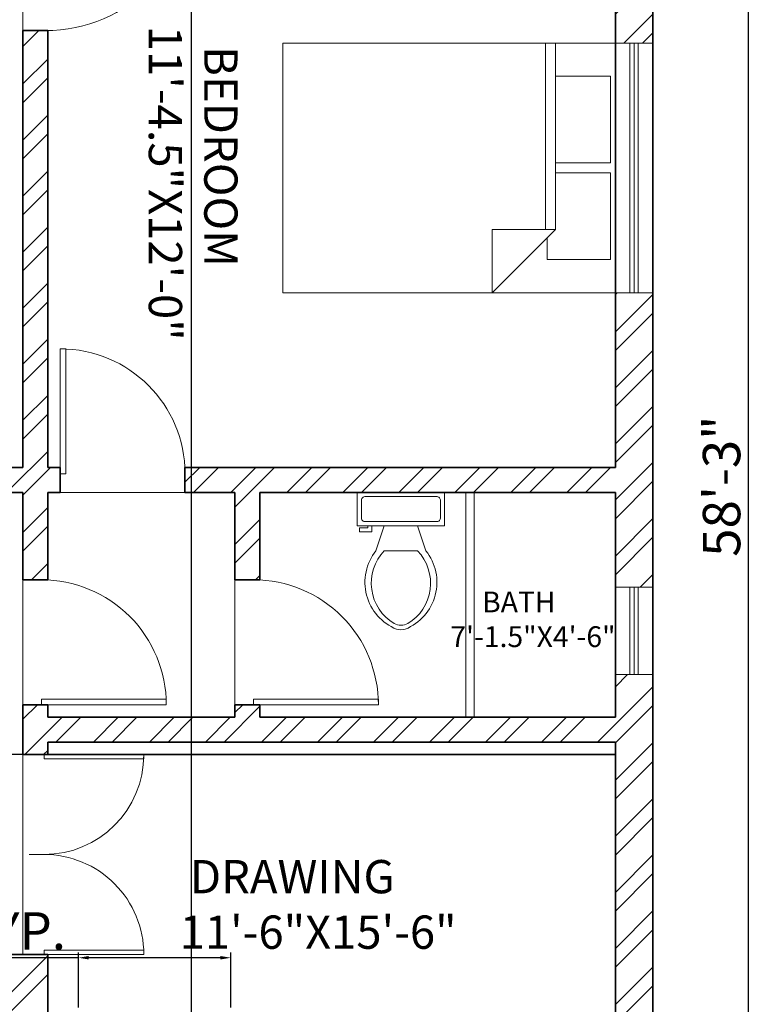
# Model space of a CAD drawing. Units: inches. Extents: x 287 to 905, y 1151 to 2037.
# Tile 4 of 5: x 646 to 822, y 1503 to 1739. Entities that reach past the tile are written whole.
import ezdxf

# ---------------------------------------------------------------- set-up
doc = ezdxf.new("R2010")
doc.units = ezdxf.units.IN
for name, color, linetype, lineweight in [('A-ANNO-DIMS', 2, 'Continuous', 18), ('A-AREA-IDEN', 7, 'Continuous', 18), ('A-DOOR', 4, 'Continuous', 18), ('A-FLOR-FIXT', 8, 'Continuous', 18), ('A-FURN', 9, 'Continuous', 18), ('A-WALL', 7, 'Continuous', 35), ('A-WALL-PATT', 252, 'Continuous', 13)]:
    doc.layers.add(name, color=color, linetype=linetype, lineweight=lineweight)
doc.layers.add('A-GLAZ', color=244, linetype='Continuous', lineweight=18, true_color=0x991b1e)
doc.layers.add('L-PLNT-PATT', color=116, linetype='Continuous', lineweight=13, true_color=0x136734)
doc.styles.get("Standard").update_dxf_attribs({"font": 'arial.ttf'})
doc.dimstyles.new('ISO-25', dxfattribs={"dimtxt": 9, "dimasz": 2.5, "dimexe": 1.25, "dimexo": 0.625, "dimtad": 1, "dimlunit": 3, "dimtxsty": 'Standard', "dimcen": 2.5, "dimadec": 0, "dimazin": 0, "dimtfac": 1, "dimtmove": 0, "dimatfit": 3, "dimfxl": 1, "dimarcsym": 0})

# ---------------------------------------------------------------- blocks, each defined once
blk = doc.blocks.new('*U2')
for p, q in [((0, 0), (0, -6)), ((40, 0), (40, -6))]:
    blk.add_line(p, q)
blk.add_lwpolyline([(0, 0), (0, 40), (1.75, 40), (1.75, 0)], close=True)
blk.add_arc((0, 0), 40, 0, 90)
blk = doc.blocks.new('*U3')
for p, q in [((0, 0), (0, -6)), ((-40, 0), (-40, -6))]:
    blk.add_line(p, q)
blk.add_lwpolyline([(0, 0), (0, 40), (-1.75, 40), (-1.75, 0)], close=True)
blk.add_arc((0, 0), 40, 90, 180)
blk = doc.blocks.new('*U6')
for p, q in [((0, 0), (0, -6)), ((40, 0), (40, -6))]:
    blk.add_line(p, q)
blk.add_lwpolyline([(0, 0), (0, 40), (1.75, 40), (1.75, 0)], close=True)
blk.add_arc((0, 0), 40, 0, 90)
blk = doc.blocks.new('Bed - Queen')
for p, q in [((0, -80.00003), (0, 0)), ((0, 0), (59.99999, 0)), ((59.99999, 0), (59.99999, -80.00003)), ((7.99999, -1.2), (28.79998, -1.2)), ((7.99999, -14.4), (7.99999, -1.2)), ((28.79998, -1.2), (28.79998, -14.4)), ((31.19999, -1.2), (51.99999, -1.2)), ((31.19999, -14.4), (31.19999, -1.2)), ((51.99999, -1.2), (51.99999, -16.4)), ((0, -14.4), (44.8, -14.4)), ((59.99999, -29.6), (44.8, -14.4)), ((44.8, -14.4), (44.8, -29.6)), ((51.99999, -16.4), (46.79936, -16.4)), ((44.8, -16.8), (0, -16.8)), ((44.8, -29.6), (59.99999, -29.6)), ((59.99999, -80.00003), (0, -80.00003))]:
    blk.add_line(p, q)
blk = doc.blocks.new('*D14')
at = {"layer": 'A-ANNO-DIMS', "color": 0, "lineweight": -2, "transparency": 16777216}
for p, q in [((798.48, 1976.83), (822.01, 1976.83)), ((820.76, 1974.33), (820.76, 1280.33)), ((798.48, 1277.83), (822.01, 1277.83))]:
    blk.add_line(p, q, dxfattribs=at)
at = {"layer": 'A-ANNO-DIMS', "color": 0, "transparency": 16777216}
for points in [[(820.35, 1974.33), (821.18, 1974.33), (820.76, 1976.83)], [(820.35, 1280.33), (821.18, 1280.33), (820.76, 1277.83)]]:
    blk.add_solid(points, dxfattribs=at)
at = {"layer": 'Defpoints', "color": 0, "transparency": 16777216}
for p in [(797.86, 1976.83), (797.86, 1277.83), (820.76, 1277.83)]:
    blk.add_point(p, dxfattribs=at)
at = {"layer": 'A-ANNO-DIMS', "color": 0, "transparency": 16777216, "insert": (815.54, 1627.33), "char_height": 9, "attachment_point": 5, "rotation": 90}
blk.add_mtext('58\'-3"', dxfattribs=at)
blk = doc.blocks.new('*U12')
for p, q in [((9.5, -6), (9.5, -2)), ((-10, -8.5), (-8, -8.5)), ((-10, -9.5), (-10, -8.5)), ((-8, -8.5), (-8, -8)), ((-7, -8), (-7, -9.5)), ((-4, -8), (-6, -14)), ((4, -8), (6, -14)), ((-7, -9.5), (-10, -9.5)), ((4, -14), (-4, -14))]:
    blk.add_line(p, q)
blk.add_lwpolyline([(10.5, -8), (10.5, 0), (-10.5, 0), (-10.5, -8)], close=True)
for points in [[(-9.5, -2), (-9.5, -6)], [(8.5, -1), (-8.5, -1)], [(-8.5, -7), (8.5, -7)]]:
    blk.add_lwpolyline(points)
for centre, radius, start, end in [((-8.62, -1.88), 0.884, 81.8699, 188.1301), ((8.62, -1.88), 0.884, 351.8699, 98.1301), ((-8.62, -6.12), 0.884, 171.8699, 278.1301), ((8.62, -6.12), 0.884, 261.8699, 8.1301), ((3.52, -21.58), 12.17, 141.4691, 247.9714), ((4.2, -21.82), 11.33, 136.3677, 238.9468), ((-3.52, -21.58), 12.17, 292.0284, 38.5307), ((-4.2, -21.82), 11.33, 301.053, 43.6321), ((0, -27.88), 4, 245.7318, 294.2682), ((0, -29), 4, 254.8605, 285.1395)]:
    blk.add_arc(centre, radius, start, end)
blk = doc.blocks.new('WIN-21IN')
for p, q in [((-10.5, 1), (10.5, 1)), ((-10.5, 0), (10.5, 0)), ((-10.5, -1), (10.5, -1))]:
    blk.add_line(p, q)
blk.add_lwpolyline([(-10.5, 4.5), (10.5, 4.5), (10.5, -4.5), (-10.5, -4.5)], close=True)
blk = doc.blocks.new('WIN-60IN')
for p, q in [((-1, 30), (-1, -30)), ((0, 30), (0, -30)), ((1, 30), (1, -30))]:
    blk.add_line(p, q)
blk.add_lwpolyline([(-4.5, 30), (4.5, 30), (4.5, -30), (-4.5, -30)], close=True)
blk = doc.blocks.new('*D25')
at = {"layer": 'A-ANNO-DIMS', "color": 0, "lineweight": -2, "transparency": 16777216}
for p, q in [((659.72, 1502.05), (659.72, 1515.27)), ((696.39, 1502.05), (696.39, 1515.27)), ((659.72, 1514.02), (580.15, 1514.02)), ((693.89, 1514.02), (662.22, 1514.02))]:
    blk.add_line(p, q, dxfattribs=at)
at = {"layer": 'A-ANNO-DIMS', "color": 0, "transparency": 16777216}
for points in [[(662.22, 1514.44), (662.22, 1513.61), (659.72, 1514.02)], [(693.89, 1514.44), (693.89, 1513.61), (696.39, 1514.02)]]:
    blk.add_solid(points, dxfattribs=at)
at = {"layer": 'Defpoints', "color": 0, "transparency": 16777216}
for p in [(659.72, 1514.02), (659.72, 1501.42), (696.39, 1501.42)]:
    blk.add_point(p, dxfattribs=at)
at = {"layer": 'A-ANNO-DIMS', "color": 0, "transparency": 16777216, "insert": (618.68, 1519.3), "char_height": 9, "attachment_point": 5}
blk.add_mtext('3\'-0 1/2" TYP.', dxfattribs=at)
blk = doc.blocks.new('*D35')
at = {"layer": 'A-ANNO-DIMS', "color": 0, "lineweight": -2, "transparency": 16777216}
for p, q in [((651.73, 1562.83), (370.73, 1562.83)), ((371.98, 1517.33), (371.98, 1560.33)), ((651.73, 1514.83), (370.73, 1514.83))]:
    blk.add_line(p, q, dxfattribs=at)
at = {"layer": 'A-ANNO-DIMS', "color": 0, "transparency": 16777216}
for points in [[(371.57, 1560.33), (372.4, 1560.33), (371.98, 1562.83)], [(371.57, 1517.33), (372.4, 1517.33), (371.98, 1514.83)]]:
    blk.add_solid(points, dxfattribs=at)
at = {"layer": 'Defpoints', "color": 0, "transparency": 16777216}
for p in [(371.98, 1562.83), (652.36, 1562.83), (652.36, 1514.83)]:
    blk.add_point(p, dxfattribs=at)
at = {"layer": 'A-ANNO-DIMS', "color": 0, "transparency": 16777216, "insert": (366.76, 1538.83), "char_height": 9, "attachment_point": 5, "rotation": 90}
blk.add_mtext('4\'-0"', dxfattribs=at)
blk = doc.blocks.new('*D37')
at = {"layer": 'A-ANNO-DIMS', "color": 0, "lineweight": -2, "transparency": 16777216}
for p, q in [((524.86, 1967.21), (524.86, 1157.65)), ((686.86, 1967.21), (686.86, 1157.65)), ((527.36, 1158.9), (684.36, 1158.9))]:
    blk.add_line(p, q, dxfattribs=at)
at = {"layer": 'A-ANNO-DIMS', "color": 0, "transparency": 16777216}
for points in [[(527.36, 1159.32), (527.36, 1158.49), (524.86, 1158.9)], [(684.36, 1159.32), (684.36, 1158.49), (686.86, 1158.9)]]:
    blk.add_solid(points, dxfattribs=at)
at = {"layer": 'Defpoints', "color": 0, "transparency": 16777216}
for p in [(524.86, 1967.83), (686.86, 1967.83), (686.86, 1158.9)]:
    blk.add_point(p, dxfattribs=at)
at = {"layer": 'A-ANNO-DIMS', "color": 0, "transparency": 16777216, "insert": (605.86, 1164.13), "char_height": 9, "attachment_point": 5}
blk.add_mtext('13\'-6"', dxfattribs=at)

msp = doc.modelspace()

# ---------------------------------------------------------------- hatches: boundary and pattern name
at = {"layer": 'A-WALL-PATT'}
h = msp.add_hatch(dxfattribs=at)
h.set_pattern_fill('ANSI32', color=256)
h.paths.add_polyline_path([(604.357, 1511.833), (519.857, 1511.833), (519.857, 1625.833), (607.357, 1625.833), (607.357, 1631.833), (510.857, 1631.833), (510.857, 1625.833), (513.857, 1625.833), (513.857, 1511.833), (496.063, 1511.833), (496.063, 1502.833), (604.357, 1502.833)])
h.paths.add_polyline_path([(652.357, 1511.833), (652.357, 1514.833), (643.357, 1514.833), (643.357, 1511.833), (640.357, 1511.833), (640.357, 1505.833), (643.357, 1505.833), (643.357, 1370.833), (690.607, 1370.833), (690.607, 1379.833), (652.357, 1379.833)])
h.paths.add_polyline_path([(797.857, 1582.055), (788.857, 1582.055), (788.857, 1571.833), (703.357, 1571.833), (703.357, 1574.833), (697.357, 1574.833), (697.357, 1571.833), (652.357, 1571.833), (652.357, 1574.833), (646.357, 1574.833), (646.357, 1562.833), (652.357, 1562.833), (652.357, 1565.833), (788.857, 1565.833), (788.857, 1379.833), (750.607, 1379.833), (750.607, 1370.833), (797.857, 1370.833)])
h.paths.add_polyline_path([(797.857, 1673.833), (788.857, 1673.833), (788.857, 1631.833), (685.357, 1631.833), (685.357, 1625.833), (697.357, 1625.833), (697.357, 1604.833), (703.357, 1604.833), (703.357, 1625.833), (788.857, 1625.833), (788.857, 1603.055), (797.857, 1603.055)])
h.paths.add_polyline_path([(797.857, 1976.833), (751.357, 1976.833), (751.357, 1967.833), (788.857, 1967.833), (788.857, 1919.833), (785.857, 1919.833), (785.857, 1913.833), (788.857, 1913.833), (788.857, 1781.833), (654.342, 1781.833), (643.328, 1792.848), (639.085, 1788.605), (645.857, 1781.833), (645.857, 1775.833), (646.357, 1775.833), (646.357, 1772.833), (652.357, 1772.833), (652.357, 1775.833), (788.857, 1775.833), (788.857, 1733.833), (797.857, 1733.833)])
h.paths.add_polyline_path([(755.857, 1919.833), (692.857, 1919.833), (692.857, 1967.833), (730.357, 1967.833), (730.357, 1976.833), (473.78, 1976.833), (473.78, 1967.833), (518.857, 1967.833), (518.857, 1919.833), (455.857, 1919.833), (455.857, 1913.833), (567.857, 1913.833), (567.857, 1919.833), (524.857, 1919.833), (524.857, 1967.833), (686.857, 1967.833), (686.857, 1919.833), (639.857, 1919.833), (639.857, 1913.833), (755.857, 1913.833)])
h.paths.add_polyline_path([(606.857, 1913.833), (609.857, 1913.833), (609.857, 1919.833), (597.857, 1919.833), (597.857, 1913.833), (600.857, 1913.833), (600.857, 1829.319), (589.842, 1818.304), (594.085, 1814.061), (600.857, 1820.833), (600.857, 1781.833), (597.857, 1781.833), (597.857, 1775.833), (609.857, 1775.833), (609.857, 1781.833), (606.857, 1781.833), (606.857, 1820.833), (613.629, 1814.061), (617.872, 1818.304), (606.857, 1829.319)])
h.paths.add_polyline_path([(652.357, 1736.833), (646.357, 1736.833), (646.357, 1631.833), (643.357, 1631.833), (643.357, 1625.833), (646.357, 1625.833), (646.357, 1604.833), (652.357, 1604.833), (652.357, 1625.833), (655.357, 1625.833), (655.357, 1631.833), (652.357, 1631.833)])
at = {"layer": 'L-PLNT-PATT'}
h = msp.add_hatch(dxfattribs=at)
h.set_pattern_fill('CROSS', color=256, scale=2)
h.paths.add_polyline_path([(788.857, 1283.833), (788.857, 1370.833), (643.357, 1370.833), (643.357, 1477.833), (594.127, 1477.833), (594.127, 1475.527, -0.1568242), (594.486, 1474.41, -1), (590.655, 1474.41, -0.1814073), (591.127, 1475.671), (591.127, 1502.833), (588.313, 1502.833), (588.313, 1283.833)])
h.paths.add_polyline_path([(640.902, 1304.954), (590.891, 1304.954), (590.891, 1328.274), (640.902, 1328.274)], flags=16)
h.paths.add_polyline_path([(638.902, 1306.954), (592.891, 1306.954), (592.891, 1326.274), (638.902, 1326.274)], flags=0)
h.paths.add_polyline_path([(640.902, 1340.02), (590.891, 1340.02), (590.891, 1363.34), (640.902, 1363.34)], flags=16)
h.paths.add_polyline_path([(638.902, 1342.02), (592.891, 1342.02), (592.891, 1361.34), (638.902, 1361.34)], flags=0)
h.paths.add_polyline_path([(640.902, 1371.662), (590.891, 1371.662), (590.891, 1394.982), (640.902, 1394.982)], flags=16)
h.paths.add_polyline_path([(638.902, 1373.662), (592.891, 1373.662), (592.891, 1392.982), (638.902, 1392.982)], flags=0)
h.paths.add_polyline_path([(640.902, 1406.128), (590.891, 1406.128), (590.891, 1429.448), (640.902, 1429.448)], flags=16)
h.paths.add_polyline_path([(638.902, 1408.128), (592.891, 1408.128), (592.891, 1427.448), (638.902, 1427.448)], flags=0)
h.paths.add_polyline_path([(640.902, 1439.308), (590.891, 1439.308), (590.891, 1462.628), (640.902, 1462.628)], flags=16)
h.paths.add_polyline_path([(638.902, 1441.308), (592.891, 1441.308), (592.891, 1460.628), (638.902, 1460.628)], flags=0)
h.paths.add_polyline_path([(678.527, 1323.107), (756.41, 1323.107), (756.41, 1352.959), (678.527, 1352.959)], flags=24)

# ---------------------------------------------------------------- linework, layer by layer
at = {"layer": 'A-DOOR'}
for p, q in [((646.357, 1772.833), (646.357, 1736.833)), ((655.357, 1625.833), (685.357, 1625.833)), ((646.357, 1604.833), (646.357, 1574.833)), ((697.357, 1574.833), (697.357, 1604.833)), ((646.357, 1562.833), (646.357, 1514.833))]:
    msp.add_line(p, q, dxfattribs=at)
at = {"layer": 'A-FLOR-FIXT'}
for p, q in [((752.857, 1625.833), (752.857, 1571.833)), ((754.857, 1625.833), (754.857, 1571.833))]:
    msp.add_line(p, q, dxfattribs=at)
at = {"layer": 'A-WALL'}
for p, q in [((797.857, 1976.833), (797.857, 1277.833)), ((788.857, 1775.833), (788.857, 1631.833)), ((646.357, 1736.833), (652.357, 1736.833)), ((646.357, 1736.833), (646.357, 1631.833)), ((652.357, 1736.833), (652.357, 1631.833)), ((643.357, 1631.833), (646.357, 1631.833)), ((652.357, 1631.833), (655.357, 1631.833)), ((655.357, 1631.833), (655.357, 1625.833)), ((685.357, 1631.833), (685.357, 1625.833)), ((685.357, 1631.833), (788.857, 1631.833)), ((643.357, 1625.833), (646.357, 1625.833)), ((646.357, 1625.833), (646.357, 1604.833)), ((652.357, 1625.833), (655.357, 1625.833)), ((652.357, 1625.833), (652.357, 1604.833)), ((685.357, 1625.833), (697.357, 1625.833)), ((697.357, 1625.833), (697.357, 1604.833)), ((703.357, 1625.833), (703.357, 1604.833)), ((703.357, 1625.833), (788.857, 1625.833)), ((788.857, 1625.833), (788.857, 1571.833)), ((652.357, 1604.833), (646.357, 1604.833)), ((703.357, 1604.833), (697.357, 1604.833)), ((646.357, 1574.833), (646.357, 1562.833)), ((652.357, 1574.833), (646.357, 1574.833)), ((646.357, 1574.833), (646.357, 1571.833)), ((652.357, 1574.833), (652.357, 1571.833)), ((703.357, 1574.833), (697.357, 1574.833)), ((697.357, 1574.833), (697.357, 1571.833)), ((703.357, 1574.833), (703.357, 1571.833)), ((652.357, 1571.833), (697.357, 1571.833)), ((703.357, 1571.833), (788.857, 1571.833)), ((652.357, 1565.833), (788.857, 1565.833)), ((652.357, 1562.833), (652.357, 1565.833)), ((788.857, 1565.833), (788.857, 1379.833)), ((646.357, 1562.833), (788.857, 1562.833)), ((643.357, 1514.833), (652.357, 1514.833)), ((652.357, 1511.833), (652.357, 1514.833)), ((652.357, 1511.833), (652.357, 1379.833))]:
    msp.add_line(p, q, dxfattribs=at)

# ---------------------------------------------------------------- block references
at = {"layer": 'A-DOOR'}
for name, p, xscale, yscale, zscale, rotation in [('*U6', (651.757, 1772.833), 0.9000000000001479, 0.9000000000001479, 0.9000000000001479, 270), ('*U3', (650.857, 1574.833), 0.7500000000000029, 0.7500000000000029, 0.7500000000000029, 270.0000000000019), ('*U3', (701.857, 1574.833), 0.7500000000000029, 0.7500000000000029, 0.7500000000000029, 270.0000000000019), ('*U3', (651.457, 1562.833), -0.5999999999999978, 0.5999999999999978, 0.5999999999999978, 269.9999999999981), ('*U3', (651.457, 1514.833), 0.5999999999999978, 0.5999999999999978, 0.5999999999999978, 270.0000000000019)]:
    msp.add_blockref(name, p, dxfattribs=dict(at, xscale=xscale, yscale=yscale, zscale=zscale, rotation=rotation))
at = {"layer": 'A-DOOR', "xscale": 0.7500000000000029, "yscale": 0.7500000000000029, "zscale": 0.7500000000000029}
msp.add_blockref('*U2', (655.357, 1630.333), dxfattribs=at)
at = {"layer": 'A-FLOR-FIXT'}
msp.add_blockref('*U12', (737.282, 1625.833), dxfattribs=at)
at = {"layer": 'A-FURN', "rotation": 269.9999999999996}
msp.add_blockref('Bed - Queen', (788.857, 1733.833), dxfattribs=at)
at = {"layer": 'A-GLAZ'}
msp.add_blockref('WIN-60IN', (793.357, 1703.833), dxfattribs=at)
at = {"layer": 'A-GLAZ', "rotation": 269.9999999999987}
msp.add_blockref('WIN-21IN', (793.357, 1592.554), dxfattribs=at)

# ---------------------------------------------------------------- texts
at = {"layer": 'A-AREA-IDEN', "insert": (697.986, 1737.977), "char_height": 8, "attachment_point": 1, "rotation": 270}
msp.add_mtext_dynamic_manual_height_columns('  BEDROOM\\P11\'-4.5"X12\'-0"', width=72.39263, gutter_width=12.5, heights=[0], dxfattribs=at)
at = {"layer": 'A-AREA-IDEN', "attachment_point": 1}
for s, width, insert, char_height in [('     BATH\\P7\'-1.5"X4\'-6"', 38.86902, (749.153, 1602.011), 5), (' DRAWING\\P11\'-6"X15\'-6"', 62.50542, (684.083, 1537.508), 8)]:
    msp.add_mtext_dynamic_manual_height_columns(s, width=width, gutter_width=12.5, heights=[0], dxfattribs=dict(at, insert=insert, char_height=char_height))

# ---------------------------------------------------------------- dimensions: what is measured, and where the dimension line sits
at = {"layer": 'A-ANNO-DIMS'}
for base, p1, p2, override, picture, middle in [((820.762, 1277.833), (797.857, 1976.833), (797.857, 1277.833), {"dimclrd": 0, "dimclre": 0, "dimclrt": 0}, '*D14', (815.538, 1627.333)), ((371.982, 1562.833), (652.357, 1514.833), (652.357, 1562.833), {"dimdec": 1, "dimlfac": 1, "dimrnd": 0, "dimzin": 1, "dimdsep": 46, "dimlunit": 4, "dimfrac": 2}, '*D35', (366.762, 1538.833))]:
    dim = msp.add_linear_dim(base=base, p1=p1, p2=p2, angle=90, dimstyle='ISO-25', override=override, dxfattribs=at)
    dim.commit()
    dim.dimension.update_dxf_attribs({"geometry": picture, "text_midpoint": middle})
dim = msp.add_linear_dim(base=(686.857, 1158.902), p1=(524.857, 1967.833), p2=(686.857, 1967.833), dimstyle='ISO-25', override={"dimdec": 1, "dimlfac": 1, "dimrnd": 0, "dimzin": 1, "dimdsep": 46, "dimlunit": 4, "dimfrac": 2}, dxfattribs=at)
dim.commit()
dim.dimension.update_dxf_attribs({"geometry": '*D37', "text_midpoint": (605.857, 1164.125)})
dim = msp.add_linear_dim(base=(659.721, 1514.022), p1=(696.388, 1501.422), p2=(659.721, 1501.422), angle=180, text='<> TYP.', dimstyle='ISO-25', override={"dimdec": 1, "dimlfac": 1, "dimrnd": 0, "dimzin": 1, "dimdsep": 46, "dimlunit": 4, "dimfrac": 2}, dxfattribs=at)
dim.commit()
dim.dimension.update_dxf_attribs({"geometry": '*D25', "text_midpoint": (618.684, 1519.304)})

doc.saveas('drawing.dxf')
